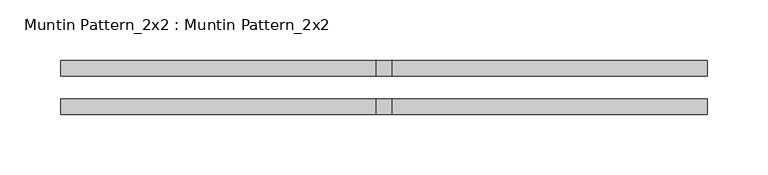
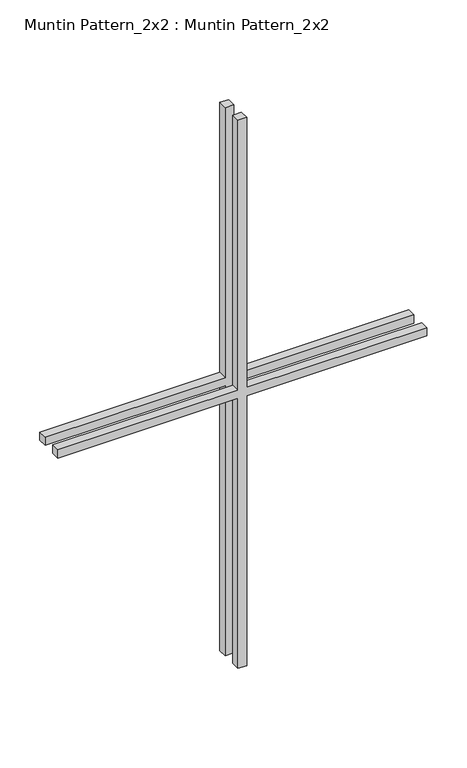
"""IFC4 building model written with IfcOpenShell, lengths in millimetres: proxy geometry, Muntin Pattern_2x2 : Muntin Pattern_2x2."""

from ifc_helpers import new_model, si_unit, frame, origin, place, context, project, spatial, polyline, outline, extrude, source, transform, mapped, element, save


def muntin_pattern_2x2_muntin_pattern_2x2_f7d54b4d(model_context):
    return source(origin(), model_context, "Body", "SweptSolid", [
        extrude(outline(polyline([(425.45, -6.35), (425.45, -266.7), (412.75, -266.7), (412.75, -6.35), (0.0, -6.35), (0.0, 6.35), (412.75, 6.35), (412.75, 266.7), (425.45, 266.7), (425.45, 6.35), (838.2, 6.35), (838.2, -6.35), (425.45, -6.35)])), frame((0.0, -22.225, 0.0), z_axis=(0.0, 1.0, 0.0), x_axis=(0.0, 0.0, 1.0)), (0.0, 0.0, 1.0), 12.7),
        extrude(outline(polyline([(425.45, -6.35), (425.45, -266.7), (412.75, -266.7), (412.75, -6.35), (0.0, -6.35), (0.0, 6.35), (412.75, 6.35), (412.75, 266.7), (425.45, 266.7), (425.45, 6.35), (838.2, 6.35), (838.2, -6.35), (425.45, -6.35)])), frame((0.0, 9.525, 0.0), z_axis=(0.0, 1.0, 0.0), x_axis=(0.0, 0.0, 1.0)), (0.0, 0.0, 1.0), 12.7),
    ])


if __name__ == "__main__":
    model = new_model("IFC4")
    model_context = context("Model", 3, world=origin())
    ifc_project = project(units=[si_unit("LENGTHUNIT", "METRE", prefix="MILLI")], contexts=[model_context])
    site = spatial("IfcSite", under=ifc_project)
    building = spatial("IfcBuilding", under=site)
    placement = place(None, origin())
    muntin_pattern_2x2_muntin_pattern_2x2_shape = muntin_pattern_2x2_muntin_pattern_2x2_f7d54b4d(model_context)
    element("IfcBuildingElementProxy", 1, Name="Muntin Pattern_2x2 : Muntin Pattern_2x2", ObjectType="Muntin Pattern_2x2 : Muntin Pattern_2x2", at=placement, inside=building, context=model_context, shape_type="MappedRepresentation", body=[
        mapped(muntin_pattern_2x2_muntin_pattern_2x2_shape, transform((0.0, 0.0, 0.0), x_axis=(1.0, 0.0, 0.0), y_axis=(0.0, 1.0, 0.0), z_axis=(0.0, 0.0, 1.0))),
    ])
    save(model, "model.ifc")

# Revit data of these elements
# Type "Muntin Pattern_2x2 : Muntin Pattern_2x2"
#   Width [instance default] = 4' - 0"
#   Thickness = 0' - 0 1/2"
#   Height [instance default] = 4' - 0"
#   Distance = 0' - 0 3/4"
#   Interior Material [instance default] = none
#   Exterior Material [instance default] = none
#   Default Elevation = 0
# Element 1 (IfcBuildingElementProxy, "Muntin Pattern_2x2 : Muntin Pattern_2x2")
#   Width = 1' - 9"
#   Height = 2' - 9"
#   Interior Material = Wood - Stained
#   Exterior Material = Clad - White
#   Materials on its faces: "Clad - White", "Wood - Stained"
# Materials
#   "Clad - White": class "Wood", colour RGB 245 245 243, transparency 0, Cost = 0
#   "Wood - Stained": class "Wood", colour RGB 173 132 96, transparency 0, Cost = 0
